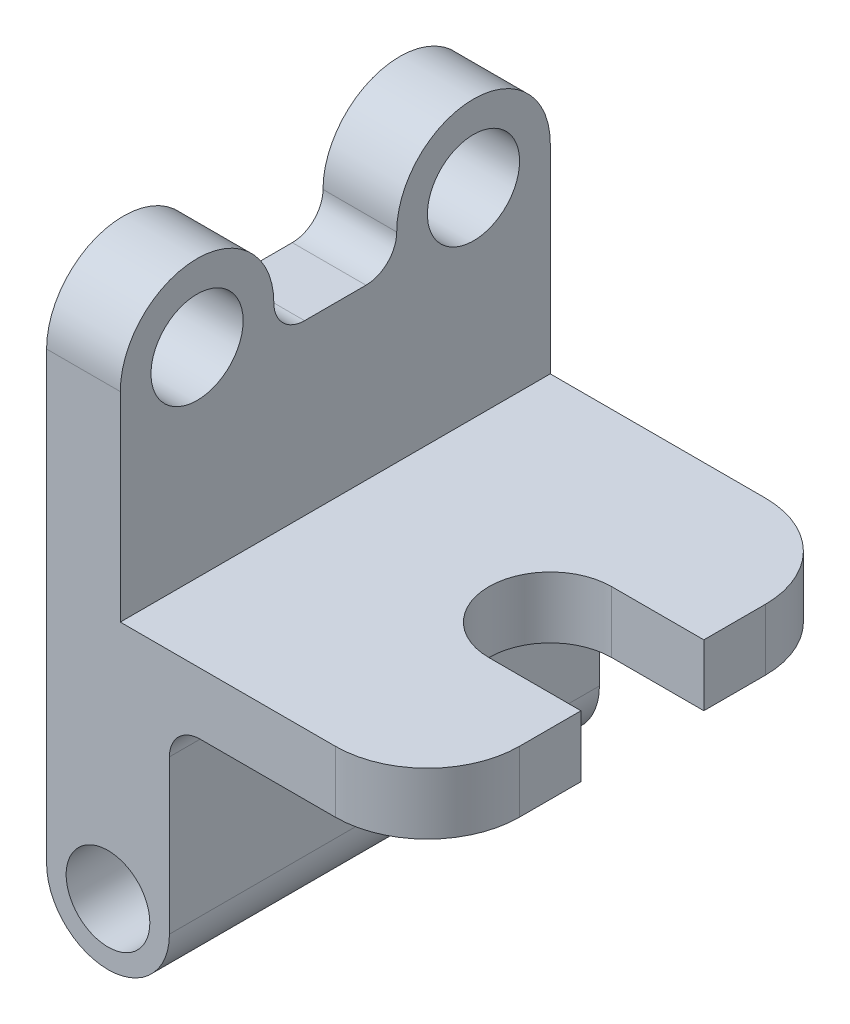
ISO-10303-21;
HEADER;
FILE_DESCRIPTION(('STEP AP214'),'2;1');
FILE_NAME('part.step','',(''),(''),'','','');
FILE_SCHEMA(('AUTOMOTIVE_DESIGN { 1 0 10303 214 1 1 1 1 }'));
ENDSEC;
DATA;
#1=APPLICATION_CONTEXT('core data for automotive mechanical design processes');
#2=APPLICATION_PROTOCOL_DEFINITION('international standard','automotive_design',2000,#1);
#3=PRODUCT_CONTEXT('',#1,'mechanical');
#4=PRODUCT('Part','Part','',(#3));
#5=PRODUCT_RELATED_PRODUCT_CATEGORY('part','',(#4));
#6=PRODUCT_DEFINITION_FORMATION('','',#4);
#7=PRODUCT_DEFINITION_CONTEXT('part definition',#1,'design');
#8=PRODUCT_DEFINITION('design','',#6,#7);
#9=PRODUCT_DEFINITION_SHAPE('','',#8);
#10=(LENGTH_UNIT() NAMED_UNIT(*) SI_UNIT(.MILLI.,.METRE.));
#11=(NAMED_UNIT(*) PLANE_ANGLE_UNIT() SI_UNIT($,.RADIAN.));
#12=(NAMED_UNIT(*) SI_UNIT($,.STERADIAN.) SOLID_ANGLE_UNIT());
#13=UNCERTAINTY_MEASURE_WITH_UNIT(LENGTH_MEASURE(1.E-05),#10,'distance_accuracy_value','');
#14=(GEOMETRIC_REPRESENTATION_CONTEXT(3) GLOBAL_UNCERTAINTY_ASSIGNED_CONTEXT((#13)) GLOBAL_UNIT_ASSIGNED_CONTEXT((#10,
#11,#12)) REPRESENTATION_CONTEXT('',''));
#15=CARTESIAN_POINT('',(0.,0.,0.));
#16=DIRECTION('',(0.,0.,1.));
#17=DIRECTION('',(1.,0.,0.));
#18=AXIS2_PLACEMENT_3D('',#15,#16,#17);
#19=CARTESIAN_POINT('',(47.,0.,-55.));
#20=DIRECTION('',(0.,-1.,0.));
#21=DIRECTION('',(0.,0.,-1.));
#22=AXIS2_PLACEMENT_3D('',#19,#20,#21);
#23=PLANE('',#22);
#24=DIRECTION('',(1.,0.,0.));
#25=VECTOR('',#24,1.);
#26=CARTESIAN_POINT('',(0.,0.,0.));
#27=LINE('',#26,#25);
#28=CARTESIAN_POINT('',(25.,0.,0.));
#29=VERTEX_POINT('',#28);
#30=CARTESIAN_POINT('',(46.9999999999999,0.,0.));
#31=VERTEX_POINT('',#30);
#32=EDGE_CURVE('E254',#29,#31,#27,.T.);
#33=ORIENTED_EDGE('',*,*,#32,.F.);
#34=DIRECTION('',(0.,0.,1.));
#35=VECTOR('',#34,1.);
#36=CARTESIAN_POINT('',(25.,0.,-70.));
#37=LINE('',#36,#35);
#38=CARTESIAN_POINT('',(25.,0.,-70.));
#39=VERTEX_POINT('',#38);
#40=EDGE_CURVE('E251',#39,#29,#37,.T.);
#41=ORIENTED_EDGE('',*,*,#40,.F.);
#42=DIRECTION('',(-1.,0.,0.));
#43=VECTOR('',#42,1.);
#44=CARTESIAN_POINT('',(0.,0.,-70.));
#45=LINE('',#44,#43);
#46=CARTESIAN_POINT('',(46.9999999999999,0.,-70.));
#47=VERTEX_POINT('',#46);
#48=EDGE_CURVE('E262',#47,#39,#45,.T.);
#49=ORIENTED_EDGE('',*,*,#48,.F.);
#50=CARTESIAN_POINT('',(47.,0.,-55.));
#51=DIRECTION('',(0.,1.,0.));
#52=DIRECTION('',(0.,0.,-1.));
#53=AXIS2_PLACEMENT_3D('',#50,#51,#52);
#54=CIRCLE('',#53,15.);
#55=CARTESIAN_POINT('',(62.,0.,-54.9999999999999));
#56=VERTEX_POINT('',#55);
#57=EDGE_CURVE('E293',#56,#47,#54,.T.);
#58=ORIENTED_EDGE('',*,*,#57,.F.);
#59=DIRECTION('',(0.,0.,-1.));
#60=VECTOR('',#59,1.);
#61=CARTESIAN_POINT('',(62.,0.,-45.));
#62=LINE('',#61,#60);
#63=CARTESIAN_POINT('',(62.,0.,-45.));
#64=VERTEX_POINT('',#63);
#65=EDGE_CURVE('E291',#64,#56,#62,.T.);
#66=ORIENTED_EDGE('',*,*,#65,.F.);
#67=DIRECTION('',(1.,0.,0.));
#68=VECTOR('',#67,1.);
#69=CARTESIAN_POINT('',(47.,0.,-45.));
#70=LINE('',#69,#68);
#71=CARTESIAN_POINT('',(47.,0.,-45.));
#72=VERTEX_POINT('',#71);
#73=EDGE_CURVE('E292',#72,#64,#70,.T.);
#74=ORIENTED_EDGE('',*,*,#73,.F.);
#75=CARTESIAN_POINT('',(47.,0.,-35.));
#76=DIRECTION('',(0.,-1.,0.));
#77=DIRECTION('',(0.,0.,1.));
#78=AXIS2_PLACEMENT_3D('',#75,#76,#77);
#79=CIRCLE('',#78,10.);
#80=CARTESIAN_POINT('',(47.,0.,-25.));
#81=VERTEX_POINT('',#80);
#82=EDGE_CURVE('E286',#81,#72,#79,.T.);
#83=ORIENTED_EDGE('',*,*,#82,.F.);
#84=DIRECTION('',(-1.,0.,0.));
#85=VECTOR('',#84,1.);
#86=CARTESIAN_POINT('',(62.,0.,-25.));
#87=LINE('',#86,#85);
#88=CARTESIAN_POINT('',(62.,0.,-25.));
#89=VERTEX_POINT('',#88);
#90=EDGE_CURVE('E290',#89,#81,#87,.T.);
#91=ORIENTED_EDGE('',*,*,#90,.F.);
#92=DIRECTION('',(0.,0.,-1.));
#93=VECTOR('',#92,1.);
#94=CARTESIAN_POINT('',(62.,0.,-15.0000000000001));
#95=LINE('',#94,#93);
#96=CARTESIAN_POINT('',(62.,0.,-15.0000000000001));
#97=VERTEX_POINT('',#96);
#98=EDGE_CURVE('E281',#97,#89,#95,.T.);
#99=ORIENTED_EDGE('',*,*,#98,.F.);
#100=CARTESIAN_POINT('',(47.,0.,-15.));
#101=DIRECTION('',(0.,1.,0.));
#102=DIRECTION('',(0.,0.,1.));
#103=AXIS2_PLACEMENT_3D('',#100,#101,#102);
#104=CIRCLE('',#103,15.);
#105=EDGE_CURVE('E283',#31,#97,#104,.T.);
#106=ORIENTED_EDGE('',*,*,#105,.F.);
#107=EDGE_LOOP('',(#33,#41,#49,#58,#66,#74,#83,#91,#99,#106));
#108=FACE_BOUND('',#107,.T.);
#109=ADVANCED_FACE('F39',(#108),#23,.T.);
#110=CARTESIAN_POINT('',(0.,10.,0.));
#111=DIRECTION('',(1.,0.,0.));
#112=DIRECTION('',(0.,0.,-1.));
#113=AXIS2_PLACEMENT_3D('',#110,#111,#112);
#114=PLANE('',#113);
#115=CARTESIAN_POINT('',(0.,42.5,-12.5));
#116=DIRECTION('',(1.,0.,0.));
#117=DIRECTION('',(0.,0.,-1.));
#118=AXIS2_PLACEMENT_3D('',#115,#116,#117);
#119=CIRCLE('',#118,7.5);
#120=CARTESIAN_POINT('',(0.,42.5,-20.));
#121=VERTEX_POINT('',#120);
#122=EDGE_CURVE('E211',#121,#121,#119,.T.);
#123=ORIENTED_EDGE('',*,*,#122,.T.);
#124=EDGE_LOOP('',(#123));
#125=FACE_BOUND('',#124,.T.);
#126=CARTESIAN_POINT('',(0.,42.5,-57.5));
#127=DIRECTION('',(1.,0.,0.));
#128=DIRECTION('',(0.,0.,-1.));
#129=AXIS2_PLACEMENT_3D('',#126,#127,#128);
#130=CIRCLE('',#129,7.5);
#131=CARTESIAN_POINT('',(0.,42.5,-65.));
#132=VERTEX_POINT('',#131);
#133=EDGE_CURVE('E587',#132,#132,#130,.T.);
#134=ORIENTED_EDGE('',*,*,#133,.T.);
#135=EDGE_LOOP('',(#134));
#136=FACE_BOUND('',#135,.T.);
#137=DIRECTION('',(0.,-1.,0.));
#138=VECTOR('',#137,1.);
#139=CARTESIAN_POINT('',(0.,10.,-70.));
#140=LINE('',#139,#138);
#141=CARTESIAN_POINT('',(0.,42.5,-70.));
#142=VERTEX_POINT('',#141);
#143=CARTESIAN_POINT('',(0.,-30.,-70.));
#144=VERTEX_POINT('',#143);
#145=EDGE_CURVE('E282',#142,#144,#140,.T.);
#146=ORIENTED_EDGE('',*,*,#145,.T.);
#147=DIRECTION('',(0.,0.,1.));
#148=VECTOR('',#147,1.);
#149=CARTESIAN_POINT('',(0.,-30.,-70.));
#150=LINE('',#149,#148);
#151=CARTESIAN_POINT('',(0.,-30.,0.));
#152=VERTEX_POINT('',#151);
#153=EDGE_CURVE('E250',#144,#152,#150,.T.);
#154=ORIENTED_EDGE('',*,*,#153,.T.);
#155=DIRECTION('',(0.,-1.,0.));
#156=VECTOR('',#155,1.);
#157=CARTESIAN_POINT('',(0.,10.,0.));
#158=LINE('',#157,#156);
#159=CARTESIAN_POINT('',(0.,42.5,0.));
#160=VERTEX_POINT('',#159);
#161=EDGE_CURVE('E11',#160,#152,#158,.T.);
#162=ORIENTED_EDGE('',*,*,#161,.F.);
#163=CARTESIAN_POINT('',(0.,42.5,-12.5));
#164=DIRECTION('',(-1.,0.,0.));
#165=DIRECTION('',(0.,0.,1.));
#166=AXIS2_PLACEMENT_3D('',#163,#164,#165);
#167=CIRCLE('',#166,12.5);
#168=CARTESIAN_POINT('',(0.,42.5,-25.));
#169=VERTEX_POINT('',#168);
#170=EDGE_CURVE('E177',#160,#169,#167,.T.);
#171=ORIENTED_EDGE('',*,*,#170,.T.);
#172=CARTESIAN_POINT('',(0.,42.5,-30.));
#173=DIRECTION('',(1.,0.,0.));
#174=DIRECTION('',(0.,0.,-1.));
#175=AXIS2_PLACEMENT_3D('',#172,#173,#174);
#176=CIRCLE('',#175,5.);
#177=CARTESIAN_POINT('',(0.,37.5,-30.));
#178=VERTEX_POINT('',#177);
#179=EDGE_CURVE('E209',#169,#178,#176,.T.);
#180=ORIENTED_EDGE('',*,*,#179,.T.);
#181=DIRECTION('',(0.,0.,-1.));
#182=VECTOR('',#181,1.);
#183=CARTESIAN_POINT('',(0.,37.5,-40.));
#184=LINE('',#183,#182);
#185=CARTESIAN_POINT('',(0.,37.5,-40.));
#186=VERTEX_POINT('',#185);
#187=EDGE_CURVE('E212',#178,#186,#184,.T.);
#188=ORIENTED_EDGE('',*,*,#187,.T.);
#189=CARTESIAN_POINT('',(0.,42.5,-40.));
#190=DIRECTION('',(1.,0.,0.));
#191=DIRECTION('',(0.,0.,1.));
#192=AXIS2_PLACEMENT_3D('',#189,#190,#191);
#193=CIRCLE('',#192,5.);
#194=CARTESIAN_POINT('',(0.,42.5,-45.));
#195=VERTEX_POINT('',#194);
#196=EDGE_CURVE('E220',#186,#195,#193,.T.);
#197=ORIENTED_EDGE('',*,*,#196,.T.);
#198=CARTESIAN_POINT('',(0.,42.5,-57.5));
#199=DIRECTION('',(-1.,0.,0.));
#200=DIRECTION('',(0.,0.,1.));
#201=AXIS2_PLACEMENT_3D('',#198,#199,#200);
#202=CIRCLE('',#201,12.5);
#203=EDGE_CURVE('E194',#195,#142,#202,.T.);
#204=ORIENTED_EDGE('',*,*,#203,.T.);
#205=EDGE_LOOP('',(#146,#154,#162,#171,#180,#188,#197,#204));
#206=FACE_BOUND('',#205,.T.);
#207=ADVANCED_FACE('F41',(#125,#136,#206),#114,.F.);
#208=CARTESIAN_POINT('',(0.,10.,0.));
#209=DIRECTION('',(0.,0.,-1.));
#210=DIRECTION('',(-1.,0.,0.));
#211=AXIS2_PLACEMENT_3D('',#208,#209,#210);
#212=PLANE('',#211);
#213=ORIENTED_EDGE('',*,*,#161,.T.);
#214=CARTESIAN_POINT('',(10.,-30.,0.));
#215=DIRECTION('',(0.,0.,1.));
#216=DIRECTION('',(1.,0.,0.));
#217=AXIS2_PLACEMENT_3D('',#214,#215,#216);
#218=CIRCLE('',#217,10.);
#219=CARTESIAN_POINT('',(20.,-30.,0.));
#220=VERTEX_POINT('',#219);
#221=EDGE_CURVE('E237',#152,#220,#218,.T.);
#222=ORIENTED_EDGE('',*,*,#221,.T.);
#223=DIRECTION('',(0.,1.,0.));
#224=VECTOR('',#223,1.);
#225=CARTESIAN_POINT('',(20.,-30.,0.));
#226=LINE('',#225,#224);
#227=CARTESIAN_POINT('',(20.,-5.00000000000003,0.));
#228=VERTEX_POINT('',#227);
#229=EDGE_CURVE('E248',#220,#228,#226,.T.);
#230=ORIENTED_EDGE('',*,*,#229,.T.);
#231=CARTESIAN_POINT('',(25.,-5.,0.));
#232=DIRECTION('',(0.,0.,-1.));
#233=DIRECTION('',(1.,0.,0.));
#234=AXIS2_PLACEMENT_3D('',#231,#232,#233);
#235=CIRCLE('',#234,5.);
#236=EDGE_CURVE('E65',#228,#29,#235,.T.);
#237=ORIENTED_EDGE('',*,*,#236,.T.);
#238=ORIENTED_EDGE('',*,*,#32,.T.);
#239=DIRECTION('',(0.,-1.,0.));
#240=VECTOR('',#239,1.);
#241=CARTESIAN_POINT('',(46.9999999999999,10.,0.));
#242=LINE('',#241,#240);
#243=CARTESIAN_POINT('',(46.9999999999999,10.,0.));
#244=VERTEX_POINT('',#243);
#245=EDGE_CURVE('E50',#244,#31,#242,.T.);
#246=ORIENTED_EDGE('',*,*,#245,.F.);
#247=DIRECTION('',(1.,0.,0.));
#248=VECTOR('',#247,1.);
#249=CARTESIAN_POINT('',(0.,10.,0.));
#250=LINE('',#249,#248);
#251=CARTESIAN_POINT('',(12.,10.,0.));
#252=VERTEX_POINT('',#251);
#253=EDGE_CURVE('E186',#252,#244,#250,.T.);
#254=ORIENTED_EDGE('',*,*,#253,.F.);
#255=DIRECTION('',(0.,1.,0.));
#256=VECTOR('',#255,1.);
#257=CARTESIAN_POINT('',(12.,10.,0.));
#258=LINE('',#257,#256);
#259=CARTESIAN_POINT('',(12.,42.5,0.));
#260=VERTEX_POINT('',#259);
#261=EDGE_CURVE('E53',#252,#260,#258,.T.);
#262=ORIENTED_EDGE('',*,*,#261,.T.);
#263=DIRECTION('',(-1.,0.,0.));
#264=VECTOR('',#263,1.);
#265=CARTESIAN_POINT('',(12.,42.5,0.));
#266=LINE('',#265,#264);
#267=EDGE_CURVE('E175',#260,#160,#266,.T.);
#268=ORIENTED_EDGE('',*,*,#267,.T.);
#269=EDGE_LOOP('',(#213,#222,#230,#237,#238,#246,#254,#262,#268));
#270=FACE_BOUND('',#269,.T.);
#271=CARTESIAN_POINT('',(10.,-30.,0.));
#272=DIRECTION('',(0.,0.,1.));
#273=DIRECTION('',(1.,0.,0.));
#274=AXIS2_PLACEMENT_3D('',#271,#272,#273);
#275=CIRCLE('',#274,6.81068387197004);
#276=CARTESIAN_POINT('',(16.81068387197,-30.,0.));
#277=VERTEX_POINT('',#276);
#278=EDGE_CURVE('E223',#277,#277,#275,.T.);
#279=ORIENTED_EDGE('',*,*,#278,.F.);
#280=EDGE_LOOP('',(#279));
#281=FACE_BOUND('',#280,.T.);
#282=ADVANCED_FACE('F190',(#270,#281),#212,.F.);
#283=CARTESIAN_POINT('',(47.,10.,-15.));
#284=DIRECTION('',(0.,-1.,0.));
#285=DIRECTION('',(0.,0.,-1.));
#286=AXIS2_PLACEMENT_3D('',#283,#284,#285);
#287=CYLINDRICAL_SURFACE('',#286,15.);
#288=ORIENTED_EDGE('',*,*,#105,.T.);
#289=DIRECTION('',(0.,-1.,0.));
#290=VECTOR('',#289,1.);
#291=CARTESIAN_POINT('',(62.,10.,-15.0000000000001));
#292=LINE('',#291,#290);
#293=CARTESIAN_POINT('',(62.,10.,-15.0000000000001));
#294=VERTEX_POINT('',#293);
#295=EDGE_CURVE('E318',#294,#97,#292,.T.);
#296=ORIENTED_EDGE('',*,*,#295,.F.);
#297=CARTESIAN_POINT('',(47.,10.,-15.));
#298=DIRECTION('',(0.,1.,0.));
#299=DIRECTION('',(0.,0.,1.));
#300=AXIS2_PLACEMENT_3D('',#297,#298,#299);
#301=CIRCLE('',#300,15.);
#302=EDGE_CURVE('E263',#244,#294,#301,.T.);
#303=ORIENTED_EDGE('',*,*,#302,.F.);
#304=ORIENTED_EDGE('',*,*,#245,.T.);
#305=EDGE_LOOP('',(#288,#296,#303,#304));
#306=FACE_BOUND('',#305,.T.);
#307=ADVANCED_FACE('F322',(#306),#287,.T.);
#308=CARTESIAN_POINT('',(62.,10.,-15.0000000000001));
#309=DIRECTION('',(-1.,0.,0.));
#310=DIRECTION('',(0.,0.,1.));
#311=AXIS2_PLACEMENT_3D('',#308,#309,#310);
#312=PLANE('',#311);
#313=ORIENTED_EDGE('',*,*,#98,.T.);
#314=DIRECTION('',(0.,-1.,0.));
#315=VECTOR('',#314,1.);
#316=CARTESIAN_POINT('',(62.,10.,-25.));
#317=LINE('',#316,#315);
#318=CARTESIAN_POINT('',(62.,10.,-25.));
#319=VERTEX_POINT('',#318);
#320=EDGE_CURVE('E312',#319,#89,#317,.T.);
#321=ORIENTED_EDGE('',*,*,#320,.F.);
#322=DIRECTION('',(0.,0.,-1.));
#323=VECTOR('',#322,1.);
#324=CARTESIAN_POINT('',(62.,10.,-15.0000000000001));
#325=LINE('',#324,#323);
#326=EDGE_CURVE('E266',#294,#319,#325,.T.);
#327=ORIENTED_EDGE('',*,*,#326,.F.);
#328=ORIENTED_EDGE('',*,*,#295,.T.);
#329=EDGE_LOOP('',(#313,#321,#327,#328));
#330=FACE_BOUND('',#329,.T.);
#331=ADVANCED_FACE('F331',(#330),#312,.F.);
#332=CARTESIAN_POINT('',(62.,10.,-25.));
#333=DIRECTION('',(0.,0.,1.));
#334=DIRECTION('',(1.,0.,0.));
#335=AXIS2_PLACEMENT_3D('',#332,#333,#334);
#336=PLANE('',#335);
#337=ORIENTED_EDGE('',*,*,#90,.T.);
#338=DIRECTION('',(0.,-1.,0.));
#339=VECTOR('',#338,1.);
#340=CARTESIAN_POINT('',(47.,10.,-25.));
#341=LINE('',#340,#339);
#342=CARTESIAN_POINT('',(47.,10.,-25.));
#343=VERTEX_POINT('',#342);
#344=EDGE_CURVE('E315',#343,#81,#341,.T.);
#345=ORIENTED_EDGE('',*,*,#344,.F.);
#346=DIRECTION('',(-1.,0.,0.));
#347=VECTOR('',#346,1.);
#348=CARTESIAN_POINT('',(62.,10.,-25.));
#349=LINE('',#348,#347);
#350=EDGE_CURVE('E268',#319,#343,#349,.T.);
#351=ORIENTED_EDGE('',*,*,#350,.F.);
#352=ORIENTED_EDGE('',*,*,#320,.T.);
#353=EDGE_LOOP('',(#337,#345,#351,#352));
#354=FACE_BOUND('',#353,.T.);
#355=ADVANCED_FACE('F338',(#354),#336,.F.);
#356=CARTESIAN_POINT('',(47.,10.,-35.));
#357=DIRECTION('',(0.,-1.,0.));
#358=DIRECTION('',(0.,0.,-1.));
#359=AXIS2_PLACEMENT_3D('',#356,#357,#358);
#360=CYLINDRICAL_SURFACE('',#359,10.);
#361=ORIENTED_EDGE('',*,*,#82,.T.);
#362=DIRECTION('',(0.,-1.,0.));
#363=VECTOR('',#362,1.);
#364=CARTESIAN_POINT('',(47.,10.,-45.));
#365=LINE('',#364,#363);
#366=CARTESIAN_POINT('',(47.,10.,-45.));
#367=VERTEX_POINT('',#366);
#368=EDGE_CURVE('E310',#367,#72,#365,.T.);
#369=ORIENTED_EDGE('',*,*,#368,.F.);
#370=CARTESIAN_POINT('',(47.,10.,-35.));
#371=DIRECTION('',(0.,-1.,0.));
#372=DIRECTION('',(0.,0.,1.));
#373=AXIS2_PLACEMENT_3D('',#370,#371,#372);
#374=CIRCLE('',#373,10.);
#375=EDGE_CURVE('E269',#343,#367,#374,.T.);
#376=ORIENTED_EDGE('',*,*,#375,.F.);
#377=ORIENTED_EDGE('',*,*,#344,.T.);
#378=EDGE_LOOP('',(#361,#369,#376,#377));
#379=FACE_BOUND('',#378,.T.);
#380=ADVANCED_FACE('F393',(#379),#360,.F.);
#381=CARTESIAN_POINT('',(47.,10.,-45.));
#382=DIRECTION('',(0.,0.,-1.));
#383=DIRECTION('',(-1.,0.,0.));
#384=AXIS2_PLACEMENT_3D('',#381,#382,#383);
#385=PLANE('',#384);
#386=ORIENTED_EDGE('',*,*,#73,.T.);
#387=DIRECTION('',(0.,-1.,0.));
#388=VECTOR('',#387,1.);
#389=CARTESIAN_POINT('',(62.,10.,-45.));
#390=LINE('',#389,#388);
#391=CARTESIAN_POINT('',(62.,10.,-45.));
#392=VERTEX_POINT('',#391);
#393=EDGE_CURVE('E308',#392,#64,#390,.T.);
#394=ORIENTED_EDGE('',*,*,#393,.F.);
#395=DIRECTION('',(1.,0.,0.));
#396=VECTOR('',#395,1.);
#397=CARTESIAN_POINT('',(47.,10.,-45.));
#398=LINE('',#397,#396);
#399=EDGE_CURVE('E275',#367,#392,#398,.T.);
#400=ORIENTED_EDGE('',*,*,#399,.F.);
#401=ORIENTED_EDGE('',*,*,#368,.T.);
#402=EDGE_LOOP('',(#386,#394,#400,#401));
#403=FACE_BOUND('',#402,.T.);
#404=ADVANCED_FACE('F392',(#403),#385,.F.);
#405=CARTESIAN_POINT('',(62.,10.,-45.));
#406=DIRECTION('',(-1.,0.,0.));
#407=DIRECTION('',(0.,0.,1.));
#408=AXIS2_PLACEMENT_3D('',#405,#406,#407);
#409=PLANE('',#408);
#410=ORIENTED_EDGE('',*,*,#65,.T.);
#411=DIRECTION('',(0.,-1.,0.));
#412=VECTOR('',#411,1.);
#413=CARTESIAN_POINT('',(62.,10.,-54.9999999999999));
#414=LINE('',#413,#412);
#415=CARTESIAN_POINT('',(62.,10.,-54.9999999999999));
#416=VERTEX_POINT('',#415);
#417=EDGE_CURVE('E304',#416,#56,#414,.T.);
#418=ORIENTED_EDGE('',*,*,#417,.F.);
#419=DIRECTION('',(0.,0.,-1.));
#420=VECTOR('',#419,1.);
#421=CARTESIAN_POINT('',(62.,10.,-45.));
#422=LINE('',#421,#420);
#423=EDGE_CURVE('E273',#392,#416,#422,.T.);
#424=ORIENTED_EDGE('',*,*,#423,.F.);
#425=ORIENTED_EDGE('',*,*,#393,.T.);
#426=EDGE_LOOP('',(#410,#418,#424,#425));
#427=FACE_BOUND('',#426,.T.);
#428=ADVANCED_FACE('F387',(#427),#409,.F.);
#429=CARTESIAN_POINT('',(47.,10.,-55.));
#430=DIRECTION('',(0.,-1.,0.));
#431=DIRECTION('',(0.,0.,-1.));
#432=AXIS2_PLACEMENT_3D('',#429,#430,#431);
#433=CYLINDRICAL_SURFACE('',#432,15.);
#434=ORIENTED_EDGE('',*,*,#57,.T.);
#435=DIRECTION('',(0.,-1.,0.));
#436=VECTOR('',#435,1.);
#437=CARTESIAN_POINT('',(46.9999999999999,10.,-70.));
#438=LINE('',#437,#436);
#439=CARTESIAN_POINT('',(46.9999999999999,10.,-70.));
#440=VERTEX_POINT('',#439);
#441=EDGE_CURVE('E296',#440,#47,#438,.T.);
#442=ORIENTED_EDGE('',*,*,#441,.F.);
#443=CARTESIAN_POINT('',(47.,10.,-55.));
#444=DIRECTION('',(0.,1.,0.));
#445=DIRECTION('',(0.,0.,-1.));
#446=AXIS2_PLACEMENT_3D('',#443,#444,#445);
#447=CIRCLE('',#446,15.);
#448=EDGE_CURVE('E277',#416,#440,#447,.T.);
#449=ORIENTED_EDGE('',*,*,#448,.F.);
#450=ORIENTED_EDGE('',*,*,#417,.T.);
#451=EDGE_LOOP('',(#434,#442,#449,#450));
#452=FACE_BOUND('',#451,.T.);
#453=ADVANCED_FACE('F381',(#452),#433,.T.);
#454=CARTESIAN_POINT('',(0.,10.,-70.));
#455=DIRECTION('',(0.,0.,1.));
#456=DIRECTION('',(1.,0.,0.));
#457=AXIS2_PLACEMENT_3D('',#454,#455,#456);
#458=PLANE('',#457);
#459=ORIENTED_EDGE('',*,*,#48,.T.);
#460=CARTESIAN_POINT('',(25.,-5.,-70.));
#461=DIRECTION('',(0.,0.,-1.));
#462=DIRECTION('',(1.,0.,0.));
#463=AXIS2_PLACEMENT_3D('',#460,#461,#462);
#464=CIRCLE('',#463,5.);
#465=CARTESIAN_POINT('',(20.,-5.00000000000003,-70.));
#466=VERTEX_POINT('',#465);
#467=EDGE_CURVE('E241',#466,#39,#464,.T.);
#468=ORIENTED_EDGE('',*,*,#467,.F.);
#469=DIRECTION('',(0.,1.,0.));
#470=VECTOR('',#469,1.);
#471=CARTESIAN_POINT('',(20.,-30.,-70.));
#472=LINE('',#471,#470);
#473=CARTESIAN_POINT('',(20.,-30.,-70.));
#474=VERTEX_POINT('',#473);
#475=EDGE_CURVE('E245',#474,#466,#472,.T.);
#476=ORIENTED_EDGE('',*,*,#475,.F.);
#477=CARTESIAN_POINT('',(10.,-30.,-70.));
#478=DIRECTION('',(0.,0.,1.));
#479=DIRECTION('',(1.,0.,0.));
#480=AXIS2_PLACEMENT_3D('',#477,#478,#479);
#481=CIRCLE('',#480,10.);
#482=EDGE_CURVE('E239',#144,#474,#481,.T.);
#483=ORIENTED_EDGE('',*,*,#482,.F.);
#484=ORIENTED_EDGE('',*,*,#145,.F.);
#485=DIRECTION('',(-1.,0.,0.));
#486=VECTOR('',#485,1.);
#487=CARTESIAN_POINT('',(12.,42.5,-70.));
#488=LINE('',#487,#486);
#489=CARTESIAN_POINT('',(12.,42.5,-70.));
#490=VERTEX_POINT('',#489);
#491=EDGE_CURVE('E225',#490,#142,#488,.T.);
#492=ORIENTED_EDGE('',*,*,#491,.F.);
#493=DIRECTION('',(0.,-1.,0.));
#494=VECTOR('',#493,1.);
#495=CARTESIAN_POINT('',(12.,10.,-70.));
#496=LINE('',#495,#494);
#497=CARTESIAN_POINT('',(12.,10.,-70.));
#498=VERTEX_POINT('',#497);
#499=EDGE_CURVE('E179',#490,#498,#496,.T.);
#500=ORIENTED_EDGE('',*,*,#499,.T.);
#501=DIRECTION('',(-1.,0.,0.));
#502=VECTOR('',#501,1.);
#503=CARTESIAN_POINT('',(0.,10.,-70.));
#504=LINE('',#503,#502);
#505=EDGE_CURVE('E279',#440,#498,#504,.T.);
#506=ORIENTED_EDGE('',*,*,#505,.F.);
#507=ORIENTED_EDGE('',*,*,#441,.T.);
#508=EDGE_LOOP('',(#459,#468,#476,#483,#484,#492,#500,#506,#507));
#509=FACE_BOUND('',#508,.T.);
#510=CARTESIAN_POINT('',(10.,-30.,-70.));
#511=DIRECTION('',(0.,0.,1.));
#512=DIRECTION('',(1.,0.,0.));
#513=AXIS2_PLACEMENT_3D('',#510,#511,#512);
#514=CIRCLE('',#513,6.81068387197004);
#515=CARTESIAN_POINT('',(16.81068387197,-30.,-70.));
#516=VERTEX_POINT('',#515);
#517=EDGE_CURVE('E234',#516,#516,#514,.T.);
#518=ORIENTED_EDGE('',*,*,#517,.T.);
#519=EDGE_LOOP('',(#518));
#520=FACE_BOUND('',#519,.T.);
#521=ADVANCED_FACE('F346',(#509,#520),#458,.F.);
#522=CARTESIAN_POINT('',(47.,10.,-55.));
#523=DIRECTION('',(0.,-1.,0.));
#524=DIRECTION('',(0.,0.,-1.));
#525=AXIS2_PLACEMENT_3D('',#522,#523,#524);
#526=PLANE('',#525);
#527=ORIENTED_EDGE('',*,*,#505,.T.);
#528=DIRECTION('',(0.,0.,1.));
#529=VECTOR('',#528,1.);
#530=CARTESIAN_POINT('',(12.,10.,-70.));
#531=LINE('',#530,#529);
#532=EDGE_CURVE('E192',#498,#252,#531,.T.);
#533=ORIENTED_EDGE('',*,*,#532,.T.);
#534=ORIENTED_EDGE('',*,*,#253,.T.);
#535=ORIENTED_EDGE('',*,*,#302,.T.);
#536=ORIENTED_EDGE('',*,*,#326,.T.);
#537=ORIENTED_EDGE('',*,*,#350,.T.);
#538=ORIENTED_EDGE('',*,*,#375,.T.);
#539=ORIENTED_EDGE('',*,*,#399,.T.);
#540=ORIENTED_EDGE('',*,*,#423,.T.);
#541=ORIENTED_EDGE('',*,*,#448,.T.);
#542=EDGE_LOOP('',(#527,#533,#534,#535,#536,#537,#538,#539,#540,#541));
#543=FACE_BOUND('',#542,.T.);
#544=ADVANCED_FACE('F345',(#543),#526,.F.);
#545=CARTESIAN_POINT('',(25.,-5.,-70.));
#546=DIRECTION('',(0.,0.,1.));
#547=DIRECTION('',(1.,0.,0.));
#548=AXIS2_PLACEMENT_3D('',#545,#546,#547);
#549=CYLINDRICAL_SURFACE('',#548,5.);
#550=ORIENTED_EDGE('',*,*,#236,.F.);
#551=DIRECTION('',(0.,0.,1.));
#552=VECTOR('',#551,1.);
#553=CARTESIAN_POINT('',(20.,-5.00000000000003,-70.));
#554=LINE('',#553,#552);
#555=EDGE_CURVE('E258',#466,#228,#554,.T.);
#556=ORIENTED_EDGE('',*,*,#555,.F.);
#557=ORIENTED_EDGE('',*,*,#467,.T.);
#558=ORIENTED_EDGE('',*,*,#40,.T.);
#559=EDGE_LOOP('',(#550,#556,#557,#558));
#560=FACE_BOUND('',#559,.T.);
#561=ADVANCED_FACE('F374',(#560),#549,.F.);
#562=CARTESIAN_POINT('',(20.,-30.,-70.));
#563=DIRECTION('',(1.,0.,0.));
#564=DIRECTION('',(0.,1.,0.));
#565=AXIS2_PLACEMENT_3D('',#562,#563,#564);
#566=PLANE('',#565);
#567=ORIENTED_EDGE('',*,*,#229,.F.);
#568=DIRECTION('',(0.,0.,1.));
#569=VECTOR('',#568,1.);
#570=CARTESIAN_POINT('',(20.,-30.,-70.));
#571=LINE('',#570,#569);
#572=EDGE_CURVE('E256',#474,#220,#571,.T.);
#573=ORIENTED_EDGE('',*,*,#572,.F.);
#574=ORIENTED_EDGE('',*,*,#475,.T.);
#575=ORIENTED_EDGE('',*,*,#555,.T.);
#576=EDGE_LOOP('',(#567,#573,#574,#575));
#577=FACE_BOUND('',#576,.T.);
#578=ADVANCED_FACE('F375',(#577),#566,.T.);
#579=CARTESIAN_POINT('',(10.,-30.,-70.));
#580=DIRECTION('',(0.,0.,1.));
#581=DIRECTION('',(1.,0.,0.));
#582=AXIS2_PLACEMENT_3D('',#579,#580,#581);
#583=CYLINDRICAL_SURFACE('',#582,10.);
#584=ORIENTED_EDGE('',*,*,#221,.F.);
#585=ORIENTED_EDGE('',*,*,#153,.F.);
#586=ORIENTED_EDGE('',*,*,#482,.T.);
#587=ORIENTED_EDGE('',*,*,#572,.T.);
#588=EDGE_LOOP('',(#584,#585,#586,#587));
#589=FACE_BOUND('',#588,.T.);
#590=ADVANCED_FACE('F369',(#589),#583,.T.);
#591=CARTESIAN_POINT('',(10.,-30.,-70.));
#592=DIRECTION('',(0.,0.,1.));
#593=DIRECTION('',(1.,0.,0.));
#594=AXIS2_PLACEMENT_3D('',#591,#592,#593);
#595=CYLINDRICAL_SURFACE('',#594,6.81068387197004);
#596=ORIENTED_EDGE('',*,*,#517,.F.);
#597=EDGE_LOOP('',(#596));
#598=FACE_BOUND('',#597,.T.);
#599=ORIENTED_EDGE('',*,*,#278,.T.);
#600=EDGE_LOOP('',(#599));
#601=FACE_BOUND('',#600,.T.);
#602=ADVANCED_FACE('F486',(#598,#601),#595,.F.);
#603=CARTESIAN_POINT('',(12.,42.5,-57.5));
#604=DIRECTION('',(-1.,0.,0.));
#605=DIRECTION('',(0.,0.,1.));
#606=AXIS2_PLACEMENT_3D('',#603,#604,#605);
#607=CYLINDRICAL_SURFACE('',#606,12.5);
#608=ORIENTED_EDGE('',*,*,#203,.F.);
#609=DIRECTION('',(-1.,0.,0.));
#610=VECTOR('',#609,1.);
#611=CARTESIAN_POINT('',(12.,42.5,-45.));
#612=LINE('',#611,#610);
#613=CARTESIAN_POINT('',(12.,42.5,-45.));
#614=VERTEX_POINT('',#613);
#615=EDGE_CURVE('E227',#614,#195,#612,.T.);
#616=ORIENTED_EDGE('',*,*,#615,.F.);
#617=CARTESIAN_POINT('',(12.,42.5,-57.5));
#618=DIRECTION('',(-1.,0.,0.));
#619=DIRECTION('',(0.,0.,1.));
#620=AXIS2_PLACEMENT_3D('',#617,#618,#619);
#621=CIRCLE('',#620,12.5);
#622=EDGE_CURVE('E204',#614,#490,#621,.T.);
#623=ORIENTED_EDGE('',*,*,#622,.T.);
#624=ORIENTED_EDGE('',*,*,#491,.T.);
#625=EDGE_LOOP('',(#608,#616,#623,#624));
#626=FACE_BOUND('',#625,.T.);
#627=ADVANCED_FACE('F353',(#626),#607,.T.);
#628=CARTESIAN_POINT('',(12.,42.5,-40.));
#629=DIRECTION('',(-1.,0.,0.));
#630=DIRECTION('',(0.,0.,1.));
#631=AXIS2_PLACEMENT_3D('',#628,#629,#630);
#632=CYLINDRICAL_SURFACE('',#631,5.);
#633=ORIENTED_EDGE('',*,*,#196,.F.);
#634=DIRECTION('',(-1.,0.,0.));
#635=VECTOR('',#634,1.);
#636=CARTESIAN_POINT('',(12.,37.5,-40.));
#637=LINE('',#636,#635);
#638=CARTESIAN_POINT('',(12.,37.5,-40.));
#639=VERTEX_POINT('',#638);
#640=EDGE_CURVE('E228',#639,#186,#637,.T.);
#641=ORIENTED_EDGE('',*,*,#640,.F.);
#642=CARTESIAN_POINT('',(12.,42.5,-40.));
#643=DIRECTION('',(1.,0.,0.));
#644=DIRECTION('',(0.,0.,1.));
#645=AXIS2_PLACEMENT_3D('',#642,#643,#644);
#646=CIRCLE('',#645,5.);
#647=EDGE_CURVE('E203',#639,#614,#646,.T.);
#648=ORIENTED_EDGE('',*,*,#647,.T.);
#649=ORIENTED_EDGE('',*,*,#615,.T.);
#650=EDGE_LOOP('',(#633,#641,#648,#649));
#651=FACE_BOUND('',#650,.T.);
#652=ADVANCED_FACE('F360',(#651),#632,.F.);
#653=CARTESIAN_POINT('',(12.,37.5,-40.));
#654=DIRECTION('',(0.,1.,0.));
#655=DIRECTION('',(0.,0.,1.));
#656=AXIS2_PLACEMENT_3D('',#653,#654,#655);
#657=PLANE('',#656);
#658=ORIENTED_EDGE('',*,*,#187,.F.);
#659=DIRECTION('',(-1.,0.,0.));
#660=VECTOR('',#659,1.);
#661=CARTESIAN_POINT('',(12.,37.5,-30.));
#662=LINE('',#661,#660);
#663=CARTESIAN_POINT('',(12.,37.5,-30.));
#664=VERTEX_POINT('',#663);
#665=EDGE_CURVE('E226',#664,#178,#662,.T.);
#666=ORIENTED_EDGE('',*,*,#665,.F.);
#667=DIRECTION('',(0.,0.,-1.));
#668=VECTOR('',#667,1.);
#669=CARTESIAN_POINT('',(12.,37.5,-40.));
#670=LINE('',#669,#668);
#671=EDGE_CURVE('E196',#664,#639,#670,.T.);
#672=ORIENTED_EDGE('',*,*,#671,.T.);
#673=ORIENTED_EDGE('',*,*,#640,.T.);
#674=EDGE_LOOP('',(#658,#666,#672,#673));
#675=FACE_BOUND('',#674,.T.);
#676=ADVANCED_FACE('F358',(#675),#657,.T.);
#677=CARTESIAN_POINT('',(12.,42.5,-30.));
#678=DIRECTION('',(-1.,0.,0.));
#679=DIRECTION('',(0.,0.,1.));
#680=AXIS2_PLACEMENT_3D('',#677,#678,#679);
#681=CYLINDRICAL_SURFACE('',#680,5.);
#682=ORIENTED_EDGE('',*,*,#179,.F.);
#683=DIRECTION('',(-1.,0.,0.));
#684=VECTOR('',#683,1.);
#685=CARTESIAN_POINT('',(12.,42.5,-25.));
#686=LINE('',#685,#684);
#687=CARTESIAN_POINT('',(12.,42.5,-25.));
#688=VERTEX_POINT('',#687);
#689=EDGE_CURVE('E180',#688,#169,#686,.T.);
#690=ORIENTED_EDGE('',*,*,#689,.F.);
#691=CARTESIAN_POINT('',(12.,42.5,-30.));
#692=DIRECTION('',(1.,0.,0.));
#693=DIRECTION('',(0.,0.,-1.));
#694=AXIS2_PLACEMENT_3D('',#691,#692,#693);
#695=CIRCLE('',#694,5.);
#696=EDGE_CURVE('E184',#688,#664,#695,.T.);
#697=ORIENTED_EDGE('',*,*,#696,.T.);
#698=ORIENTED_EDGE('',*,*,#665,.T.);
#699=EDGE_LOOP('',(#682,#690,#697,#698));
#700=FACE_BOUND('',#699,.T.);
#701=ADVANCED_FACE('F361',(#700),#681,.F.);
#702=CARTESIAN_POINT('',(12.,42.5,-12.5));
#703=DIRECTION('',(-1.,0.,0.));
#704=DIRECTION('',(0.,0.,1.));
#705=AXIS2_PLACEMENT_3D('',#702,#703,#704);
#706=CYLINDRICAL_SURFACE('',#705,12.5);
#707=ORIENTED_EDGE('',*,*,#170,.F.);
#708=ORIENTED_EDGE('',*,*,#267,.F.);
#709=CARTESIAN_POINT('',(12.,42.5,-12.5));
#710=DIRECTION('',(-1.,0.,0.));
#711=DIRECTION('',(0.,0.,1.));
#712=AXIS2_PLACEMENT_3D('',#709,#710,#711);
#713=CIRCLE('',#712,12.5);
#714=EDGE_CURVE('E174',#260,#688,#713,.T.);
#715=ORIENTED_EDGE('',*,*,#714,.T.);
#716=ORIENTED_EDGE('',*,*,#689,.T.);
#717=EDGE_LOOP('',(#707,#708,#715,#716));
#718=FACE_BOUND('',#717,.T.);
#719=ADVANCED_FACE('F173',(#718),#706,.T.);
#720=CARTESIAN_POINT('',(12.,42.5,-12.5));
#721=DIRECTION('',(-1.,0.,0.));
#722=DIRECTION('',(0.,0.,1.));
#723=AXIS2_PLACEMENT_3D('',#720,#721,#722);
#724=PLANE('',#723);
#725=CARTESIAN_POINT('',(12.,42.5,-12.5));
#726=DIRECTION('',(1.,0.,0.));
#727=DIRECTION('',(0.,0.,-1.));
#728=AXIS2_PLACEMENT_3D('',#725,#726,#727);
#729=CIRCLE('',#728,7.5);
#730=CARTESIAN_POINT('',(12.,42.5,-20.));
#731=VERTEX_POINT('',#730);
#732=EDGE_CURVE('E584',#731,#731,#729,.T.);
#733=ORIENTED_EDGE('',*,*,#732,.F.);
#734=EDGE_LOOP('',(#733));
#735=FACE_BOUND('',#734,.T.);
#736=CARTESIAN_POINT('',(12.,42.5,-57.5));
#737=DIRECTION('',(1.,0.,0.));
#738=DIRECTION('',(0.,0.,-1.));
#739=AXIS2_PLACEMENT_3D('',#736,#737,#738);
#740=CIRCLE('',#739,7.5);
#741=CARTESIAN_POINT('',(12.,42.5,-65.));
#742=VERTEX_POINT('',#741);
#743=EDGE_CURVE('E588',#742,#742,#740,.T.);
#744=ORIENTED_EDGE('',*,*,#743,.F.);
#745=EDGE_LOOP('',(#744));
#746=FACE_BOUND('',#745,.T.);
#747=ORIENTED_EDGE('',*,*,#532,.F.);
#748=ORIENTED_EDGE('',*,*,#499,.F.);
#749=ORIENTED_EDGE('',*,*,#622,.F.);
#750=ORIENTED_EDGE('',*,*,#647,.F.);
#751=ORIENTED_EDGE('',*,*,#671,.F.);
#752=ORIENTED_EDGE('',*,*,#696,.F.);
#753=ORIENTED_EDGE('',*,*,#714,.F.);
#754=ORIENTED_EDGE('',*,*,#261,.F.);
#755=EDGE_LOOP('',(#747,#748,#749,#750,#751,#752,#753,#754));
#756=FACE_BOUND('',#755,.T.);
#757=ADVANCED_FACE('F182',(#735,#746,#756),#724,.F.);
#758=CARTESIAN_POINT('',(0.,42.5,-57.5));
#759=DIRECTION('',(1.,0.,0.));
#760=DIRECTION('',(0.,0.,-1.));
#761=AXIS2_PLACEMENT_3D('',#758,#759,#760);
#762=CYLINDRICAL_SURFACE('',#761,7.5);
#763=ORIENTED_EDGE('',*,*,#133,.F.);
#764=EDGE_LOOP('',(#763));
#765=FACE_BOUND('',#764,.T.);
#766=ORIENTED_EDGE('',*,*,#743,.T.);
#767=EDGE_LOOP('',(#766));
#768=FACE_BOUND('',#767,.T.);
#769=ADVANCED_FACE('F526',(#765,#768),#762,.F.);
#770=CARTESIAN_POINT('',(0.,42.5,-12.5));
#771=DIRECTION('',(1.,0.,0.));
#772=DIRECTION('',(0.,0.,-1.));
#773=AXIS2_PLACEMENT_3D('',#770,#771,#772);
#774=CYLINDRICAL_SURFACE('',#773,7.5);
#775=ORIENTED_EDGE('',*,*,#122,.F.);
#776=EDGE_LOOP('',(#775));
#777=FACE_BOUND('',#776,.T.);
#778=ORIENTED_EDGE('',*,*,#732,.T.);
#779=EDGE_LOOP('',(#778));
#780=FACE_BOUND('',#779,.T.);
#781=ADVANCED_FACE('F538',(#777,#780),#774,.F.);
#782=CLOSED_SHELL('',(#109,#207,#282,#307,#331,#355,#380,#404,#428,#453,#521,#544,#561,#578,
#590,#602,#627,#652,#676,#701,#719,#757,#769,#781));
#783=MANIFOLD_SOLID_BREP('B2',#782);
#784=ADVANCED_BREP_SHAPE_REPRESENTATION('',(#18,#783),#14);
#785=SHAPE_DEFINITION_REPRESENTATION(#9,#784);
ENDSEC;
END-ISO-10303-21;
